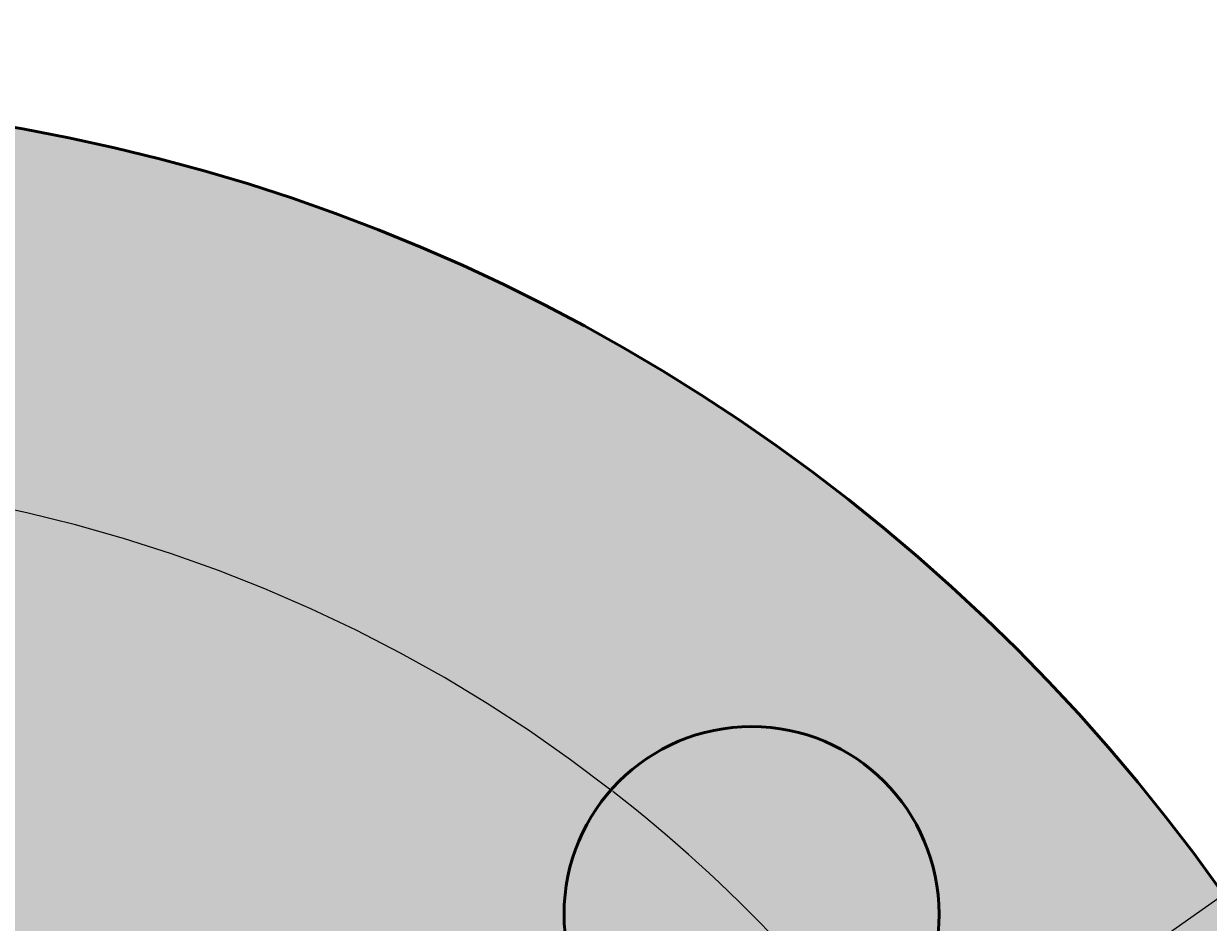
# Model space of a CAD drawing. Units: inches. Extents: x 139261 to 139415, y 52839 to 52963.
# Tile 19 of 20: x 139349 to 139381, y 52928 to 52952. Entities that reach past the tile are written whole.
import ezdxf

# ---------------------------------------------------------------- set-up
doc = ezdxf.new("R2010")
doc.units = ezdxf.units.IN
doc.header["$MEASUREMENT"] = 0
doc.linetypes.add('CENTER', pattern=[50.8, 31.75, -6.35, 6.35, -6.35])
for name, color, linetype, lineweight in [('M-CNTR', 4, 'CENTER', 18), ('M-DIMS', 2, 'Continuous', 25), ('M-HATC', 8, 'Continuous', 18), ('M-OUTL', 7, 'Continuous', 50)]:
    doc.layers.add(name, color=color, linetype=linetype, lineweight=lineweight)
doc.styles.get("Standard").update_dxf_attribs({"font": 'arial.ttf'})
doc.dimstyles.get("Standard").update_dxf_attribs({"dimtxt": 0.18, "dimasz": 0.18, "dimexe": 0.18, "dimexo": 0.0625, "dimgap": 0.09, "dimtad": 0, "dimtih": 1, "dimtoh": 1, "dimdec": 4, "dimzin": 0, "dimdsep": 46, "dimtxsty": 'Standard', "dimcen": 0.09, "dimadec": 0, "dimazin": 0, "dimtfac": 1, "dimtdec": 4, "dimtofl": 0, "dimtmove": 0, "dimatfit": 3, "dimfxl": 1, "dimtolj": 1, "dimtzin": 0, "dimarcsym": 0})

# ---------------------------------------------------------------- blocks, each defined once
blk = doc.blocks.new('*U1')
blk.add_circle((0, 0), 5)
blk = doc.blocks.new('*U2')
at = {"layer": 'M-OUTL', "color": 0, "linetype": 'ByBlock', "lineweight": -2, "transparency": 16777216, "rotation": 315}
blk.add_blockref('*U1', (139368.641, 52928.502), dxfattribs=at)
blk = doc.blocks.new('*D4')
at = {"layer": 'Defpoints', "color": 0, "transparency": 16777216}
for p in [(139373.053, 52923.26), (139307.661, 52877.175)]:
    blk.add_point(p, dxfattribs=at)
at = {"layer": 'M-DIMS', "color": 0, "lineweight": -2, "transparency": 16777216}
for p, q in [((139414.011, 52952.126), (139373.2, 52923.364)), ((139414.191, 52952.126), (139414.011, 52952.126)), ((139340.357, 52900.127), (139340.357, 52900.307)), ((139340.267, 52900.217), (139340.447, 52900.217))]:
    blk.add_line(p, q, dxfattribs=at)
blk.add_arc((139340.357, 52900.217), 40, 34.9168, 52.0771, dxfattribs=at)
at = {"layer": 'M-DIMS', "color": 0, "transparency": 16777216}
blk.add_solid([(139373.183, 52923.388), (139373.217, 52923.339), (139373.053, 52923.26)], dxfattribs=at)
at = {"layer": 'M-DIMS', "color": 0, "transparency": 16777216, "insert": (139414.822, 52952.126), "char_height": 0.18, "attachment_point": 5}
blk.add_mtext('\\A1;∅80.0000', dxfattribs=at)
blk = doc.blocks.new('*D9')
at = {"layer": 'Defpoints', "color": 0, "transparency": 16777216}
for p in [(139302.054, 52932.357), (139378.659, 52868.078)]:
    blk.add_point(p, dxfattribs=at)
at = {"layer": 'M-DIMS', "color": 0, "lineweight": -2, "transparency": 16777216}
for p, q in [((139278.893, 52951.64), (139279.073, 52951.64)), ((139279.073, 52951.64), (139301.916, 52932.472)), ((139340.357, 52900.127), (139340.357, 52900.307)), ((139340.267, 52900.217), (139340.447, 52900.217))]:
    blk.add_line(p, q, dxfattribs=at)
at = {"layer": 'M-DIMS', "color": 0, "transparency": 16777216}
blk.add_solid([(139301.936, 52932.495), (139301.897, 52932.449), (139302.054, 52932.357)], dxfattribs=at)
at = {"layer": 'M-DIMS', "color": 0, "transparency": 16777216, "insert": (139278.506, 52951.64), "char_height": 0.18, "attachment_point": 5}
blk.add_mtext('\\A1;∅100', dxfattribs=at)
blk = doc.blocks.new('*D10')
at = {"layer": 'Defpoints', "color": 0, "transparency": 16777216}
for p in [(139325.07, 52937.181), (139355.644, 52863.254)]:
    blk.add_point(p, dxfattribs=at)
at = {"layer": 'M-DIMS', "color": 0, "lineweight": -2, "transparency": 16777216}
for p, q in [((139340.357, 52900.127), (139340.357, 52900.307)), ((139340.267, 52900.217), (139340.447, 52900.217)), ((139364.816, 52841.075), (139355.712, 52863.087)), ((139364.996, 52841.075), (139364.816, 52841.075))]:
    blk.add_line(p, q, dxfattribs=at)
at = {"layer": 'M-DIMS', "color": 0, "transparency": 16777216}
blk.add_solid([(139355.74, 52863.099), (139355.685, 52863.076), (139355.644, 52863.254)], dxfattribs=at)
at = {"layer": 'M-DIMS', "color": 0, "transparency": 16777216, "insert": (139365.312, 52841.075), "char_height": 0.18, "attachment_point": 5}
blk.add_mtext('\\A1;∅80', dxfattribs=at)

msp = doc.modelspace()

# ---------------------------------------------------------------- hatches: boundary and pattern name
at = {"layer": 'M-HATC'}
h = msp.add_hatch(color=256, dxfattribs=at)
h.dxf.hatch_style = 1
h.paths.add_polyline_path([(139290.35689, 52900.21749, 1), (139390.35689, 52900.21749, 1)])
h.paths.add_polyline_path([(139335.36666, 52939.90499, -0.01563646), (139335.35689, 52940.21749, -1), (139345.35689, 52940.21749, -0.01563646), (139345.34711, 52939.90499, -0.13461315), (139364.89157, 52931.80941, -0.691035), (139373.64116, 52928.50176, -0.21521822), (139371.94881, 52924.75216, -0.13461315), (139380.04439, 52905.20771, -0.43265224), (139385.35689, 52900.21749, -0.43265224), (139380.04439, 52895.22726, -0.13461315), (139371.94881, 52875.68281, -0.21521822), (139373.64116, 52871.93321, -0.691035), (139364.89157, 52868.62556, -0.13461315), (139345.34711, 52860.52999, -0.01563646), (139345.35689, 52860.21749, -1), (139335.35689, 52860.21749, -0.01563646), (139335.36666, 52860.52999, -0.13461315), (139315.82221, 52868.62556, -0.691035), (139307.07262, 52871.93321, -0.21521822), (139308.76496, 52875.68281, -0.13461315), (139300.66939, 52895.22726, -0.43265224), (139295.35689, 52900.21749, -0.43265224), (139300.66939, 52905.20771, -0.13461315), (139308.76496, 52924.75216, -0.21521822), (139307.07262, 52928.50176, -0.691035), (139315.82221, 52931.80941, -0.13461315)], flags=16)
h.paths.add_polyline_path([(139365.35689, 52900.21749, -1), (139315.35689, 52900.21749, -1)], flags=0)
h.paths.add_polyline_path([(139323.71474, 52911.30978), (139356.99903, 52911.30978, -0.3027197), (139356.99903, 52889.12519), (139323.71474, 52889.12519, -0.3027197)], flags=0)
h.paths.add_polyline_path([(139364.89157, 52931.80941, 0.13461315), (139345.34711, 52939.90499, -0.93933644), (139335.36666, 52939.90499, 0.13461315), (139315.82221, 52931.80941, -0.18270763), (139317.07262, 52928.50176, -0.64579494), (139308.76496, 52924.75216, 0.13461315), (139300.66939, 52905.20771, -0.39601219), (139305.35689, 52900.21749, -0.39601219), (139300.66939, 52895.22726, 0.13461315), (139308.76496, 52875.68281, -0.64579494), (139317.07262, 52871.93321, -0.18270763), (139315.82221, 52868.62556, 0.13461315), (139335.36666, 52860.52999, -0.93933644), (139345.34711, 52860.52999, 0.13461315), (139364.89157, 52868.62556, -0.18270763), (139363.64116, 52871.93321, -0.64579494), (139371.94881, 52875.68281, 0.13461315), (139380.04439, 52895.22726, -0.39601219), (139375.35689, 52900.21749, -0.39601219), (139380.04439, 52905.20771, 0.13461315), (139371.94881, 52924.75216, -0.64579494), (139363.64116, 52928.50176, -0.18270763)], flags=0)
h = msp.add_hatch(color=256, dxfattribs=at)
h.dxf.hatch_style = 1
h.set_gradient(color1=(205, 105, 40), tint=1)
h.paths.add_polyline_path([(139335.35689, 52940.21749, 1), (139345.35689, 52940.21749, 1)])
h.paths.add_polyline_path([(139307.07262, 52928.50176, 1), (139317.07262, 52928.50176, 1)])
h.paths.add_polyline_path([(139295.35689, 52900.21749, 1), (139305.35689, 52900.21749, 1)])
h.paths.add_polyline_path([(139307.07262, 52871.93321, 1), (139317.07262, 52871.93321, 1)])
h.paths.add_polyline_path([(139345.35689, 52860.21749, 1), (139335.35689, 52860.21749, 1)])
h.paths.add_polyline_path([(139363.64116, 52871.93321, 1), (139373.64116, 52871.93321, 1)])
h.paths.add_polyline_path([(139375.35689, 52900.21749, 1), (139385.35689, 52900.21749, 1)])
h.paths.add_polyline_path([(139363.64116, 52928.50176, 1), (139373.64116, 52928.50176, 1)])
h = msp.add_hatch(color=256, dxfattribs=at)
h.dxf.hatch_style = 1
h.paths.add_polyline_path([(139345.34711, 52939.90499, -0.93933644), (139335.36666, 52939.90499, 0.13461315), (139315.82221, 52931.80941, -0.18270763), (139317.07262, 52928.50176, -0.64579494), (139308.76496, 52924.75216, 0.13461315), (139300.66939, 52905.20771, -0.39601219), (139305.35689, 52900.21749, -0.39601219), (139300.66939, 52895.22726, 0.13461315), (139308.76496, 52875.68281, -0.64579494), (139317.07262, 52871.93321, -0.18270763), (139315.82221, 52868.62556, 0.13461315), (139335.36666, 52860.52999, -0.93933644), (139345.34711, 52860.52999, 0.13461315), (139364.89157, 52868.62556, -0.18270763), (139363.64116, 52871.93321, -0.64579494), (139371.94881, 52875.68281, 0.13461315), (139380.04439, 52895.22726, -0.39601219), (139375.35689, 52900.21749, -0.39601219), (139380.04439, 52905.20771, 0.13461315), (139371.94881, 52924.75216, -0.64579494), (139363.64116, 52928.50176, -0.18270763), (139364.89157, 52931.80941, 0.13461315)])
h.paths.add_polyline_path([(139365.35689, 52900.21749, -1), (139315.35689, 52900.21749, -1)], flags=16)
h.paths.add_polyline_path([(139356.99903, 52911.30978, -0.3027197), (139356.99903, 52889.12519), (139323.71474, 52889.12519, -0.3027197), (139323.71474, 52911.30978)], flags=0)

# ---------------------------------------------------------------- linework, layer by layer
at = {"layer": 'M-CNTR'}
msp.add_arc((139340.35689, 52900.21749), 40, 52.166643, 82.833357, dxfattribs=at)
at = {"layer": 'M-OUTL'}
msp.add_circle((139340.35689, 52900.21749), 50, dxfattribs=at)

# ---------------------------------------------------------------- block references
msp.add_blockref('*U2', (0, 0), dxfattribs=at)

# ---------------------------------------------------------------- dimensions: what is measured, and where the dimension line sits
at = {"layer": 'M-DIMS'}
for p1, p2, override, picture, middle in [((139307.66087, 52877.17469), (139373.0529, 52923.26028), {"dimclrd": 0, "dimclre": 0, "dimclrt": 0}, '*D4', (139414.82217, 52952.12585)), ((139378.65939, 52868.07845), (139302.05438, 52932.35652), {"dimdec": 0, "dimlfac": 1, "dimrnd": 0, "dimzin": 0, "dimdsep": 46, "dimlunit": 2}, '*D9', (139278.50641, 52951.63995)), ((139325.07023, 52937.18123), (139355.64354, 52863.25374), {"dimdec": 0, "dimlfac": 1, "dimrnd": 0, "dimzin": 0, "dimdsep": 46, "dimlunit": 2}, '*D10', (139365.31206, 52841.0755))]:
    dim = msp.add_diameter_dim_2p(p1=p1, p2=p2, dimstyle='Standard', override=override, dxfattribs=at)
    dim.commit()
    dim.dimension.update_dxf_attribs({"geometry": picture, "text_midpoint": middle, "dimtype": 163})

doc.saveas('drawing.dxf')
